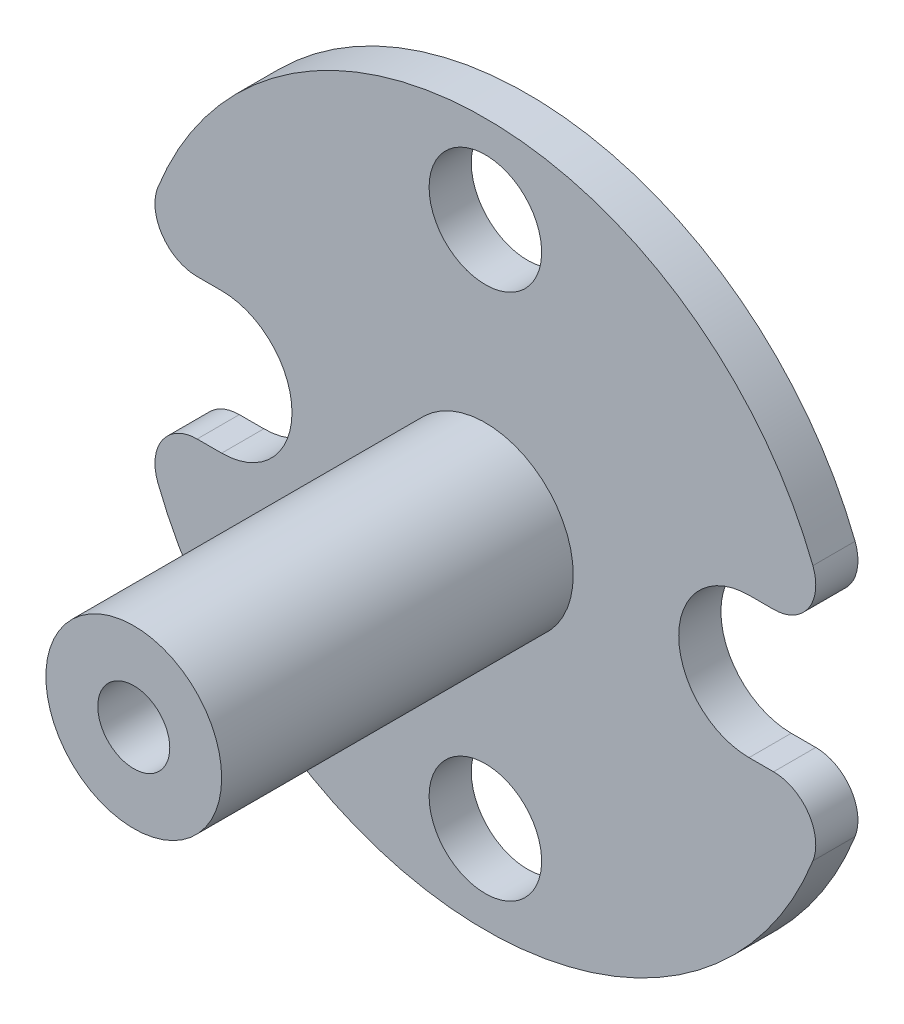
ISO-10303-21;
HEADER;
FILE_DESCRIPTION(('STEP AP214'),'2;1');
FILE_NAME('part.step','',(''),(''),'','','');
FILE_SCHEMA(('AUTOMOTIVE_DESIGN { 1 0 10303 214 1 1 1 1 }'));
ENDSEC;
DATA;
#1=APPLICATION_CONTEXT('core data for automotive mechanical design processes');
#2=APPLICATION_PROTOCOL_DEFINITION('international standard','automotive_design',2000,#1);
#3=PRODUCT_CONTEXT('',#1,'mechanical');
#4=PRODUCT('Part','Part','',(#3));
#5=PRODUCT_RELATED_PRODUCT_CATEGORY('part','',(#4));
#6=PRODUCT_DEFINITION_FORMATION('','',#4);
#7=PRODUCT_DEFINITION_CONTEXT('part definition',#1,'design');
#8=PRODUCT_DEFINITION('design','',#6,#7);
#9=PRODUCT_DEFINITION_SHAPE('','',#8);
#10=(LENGTH_UNIT() NAMED_UNIT(*) SI_UNIT(.MILLI.,.METRE.));
#11=(NAMED_UNIT(*) PLANE_ANGLE_UNIT() SI_UNIT($,.RADIAN.));
#12=(NAMED_UNIT(*) SI_UNIT($,.STERADIAN.) SOLID_ANGLE_UNIT());
#13=UNCERTAINTY_MEASURE_WITH_UNIT(LENGTH_MEASURE(1.E-05),#10,'distance_accuracy_value','');
#14=(GEOMETRIC_REPRESENTATION_CONTEXT(3) GLOBAL_UNCERTAINTY_ASSIGNED_CONTEXT((#13)) GLOBAL_UNIT_ASSIGNED_CONTEXT((#10,
#11,#12)) REPRESENTATION_CONTEXT('',''));
#15=CARTESIAN_POINT('',(0.,0.,0.));
#16=DIRECTION('',(0.,0.,1.));
#17=DIRECTION('',(1.,0.,0.));
#18=AXIS2_PLACEMENT_3D('',#15,#16,#17);
#19=CARTESIAN_POINT('',(-19.05,0.,3.048));
#20=DIRECTION('',(0.,0.,1.));
#21=DIRECTION('',(1.,0.,0.));
#22=AXIS2_PLACEMENT_3D('',#19,#20,#21);
#23=PLANE('',#22);
#24=CARTESIAN_POINT('',(0.,0.,3.048));
#25=DIRECTION('',(0.,0.,1.));
#26=DIRECTION('',(1.,0.,0.));
#27=AXIS2_PLACEMENT_3D('',#24,#25,#26);
#28=CIRCLE('',#27,6.35);
#29=CARTESIAN_POINT('',(6.35,0.,3.048));
#30=VERTEX_POINT('',#29);
#31=EDGE_CURVE('E147',#30,#30,#28,.T.);
#32=ORIENTED_EDGE('',*,*,#31,.F.);
#33=EDGE_LOOP('',(#32));
#34=FACE_BOUND('',#33,.T.);
#35=CARTESIAN_POINT('',(0.,19.05,3.048));
#36=DIRECTION('',(0.,0.,1.));
#37=DIRECTION('',(1.,0.,0.));
#38=AXIS2_PLACEMENT_3D('',#35,#36,#37);
#39=CIRCLE('',#38,4.065);
#40=CARTESIAN_POINT('',(-4.065,19.05,3.048));
#41=VERTEX_POINT('',#40);
#42=EDGE_CURVE('E168',#41,#41,#39,.T.);
#43=ORIENTED_EDGE('',*,*,#42,.F.);
#44=EDGE_LOOP('',(#43));
#45=FACE_BOUND('',#44,.T.);
#46=CARTESIAN_POINT('',(0.,0.,3.048));
#47=DIRECTION('',(0.,0.,1.));
#48=DIRECTION('',(1.,0.,0.));
#49=AXIS2_PLACEMENT_3D('',#46,#47,#48);
#50=CIRCLE('',#49,25.4);
#51=CARTESIAN_POINT('',(-23.6611408595794,-9.23636363636363,3.048));
#52=VERTEX_POINT('',#51);
#53=CARTESIAN_POINT('',(23.6611408595794,-9.23636363636363,3.048));
#54=VERTEX_POINT('',#53);
#55=EDGE_CURVE('E177',#52,#54,#50,.T.);
#56=ORIENTED_EDGE('',*,*,#55,.T.);
#57=CARTESIAN_POINT('',(20.8218039564299,-8.128,3.048));
#58=DIRECTION('',(0.,0.,1.));
#59=DIRECTION('',(1.,0.,0.));
#60=AXIS2_PLACEMENT_3D('',#57,#58,#59);
#61=CIRCLE('',#60,3.048);
#62=CARTESIAN_POINT('',(20.8218039564299,-5.08,3.048));
#63=VERTEX_POINT('',#62);
#64=EDGE_CURVE('E242',#54,#63,#61,.T.);
#65=ORIENTED_EDGE('',*,*,#64,.T.);
#66=DIRECTION('',(-1.,0.,0.));
#67=VECTOR('',#66,1.);
#68=CARTESIAN_POINT('',(19.05,-5.08,3.048));
#69=LINE('',#68,#67);
#70=CARTESIAN_POINT('',(19.05,-5.08,3.048));
#71=VERTEX_POINT('',#70);
#72=EDGE_CURVE('E185',#63,#71,#69,.T.);
#73=ORIENTED_EDGE('',*,*,#72,.T.);
#74=CARTESIAN_POINT('',(19.05,0.,3.048));
#75=DIRECTION('',(0.,0.,-1.));
#76=DIRECTION('',(-1.,0.,0.));
#77=AXIS2_PLACEMENT_3D('',#74,#75,#76);
#78=CIRCLE('',#77,5.08);
#79=CARTESIAN_POINT('',(19.05,5.08,3.048));
#80=VERTEX_POINT('',#79);
#81=EDGE_CURVE('E183',#71,#80,#78,.T.);
#82=ORIENTED_EDGE('',*,*,#81,.T.);
#83=DIRECTION('',(1.,0.,0.));
#84=VECTOR('',#83,1.);
#85=CARTESIAN_POINT('',(19.05,5.08,3.048));
#86=LINE('',#85,#84);
#87=CARTESIAN_POINT('',(20.8218039564299,5.08,3.048));
#88=VERTEX_POINT('',#87);
#89=EDGE_CURVE('E187',#80,#88,#86,.T.);
#90=ORIENTED_EDGE('',*,*,#89,.T.);
#91=CARTESIAN_POINT('',(20.8218039564299,8.128,3.048));
#92=DIRECTION('',(0.,0.,1.));
#93=DIRECTION('',(1.,0.,0.));
#94=AXIS2_PLACEMENT_3D('',#91,#92,#93);
#95=CIRCLE('',#94,3.048);
#96=CARTESIAN_POINT('',(23.6611408595794,9.23636363636363,3.048));
#97=VERTEX_POINT('',#96);
#98=EDGE_CURVE('E245',#88,#97,#95,.T.);
#99=ORIENTED_EDGE('',*,*,#98,.T.);
#100=CARTESIAN_POINT('',(0.,0.,3.048));
#101=DIRECTION('',(0.,0.,1.));
#102=DIRECTION('',(1.,0.,0.));
#103=AXIS2_PLACEMENT_3D('',#100,#101,#102);
#104=CIRCLE('',#103,25.4);
#105=CARTESIAN_POINT('',(-23.6611408595794,9.23636363636363,3.048));
#106=VERTEX_POINT('',#105);
#107=EDGE_CURVE('E186',#97,#106,#104,.T.);
#108=ORIENTED_EDGE('',*,*,#107,.T.);
#109=CARTESIAN_POINT('',(-20.8218039564299,8.128,3.048));
#110=DIRECTION('',(0.,0.,1.));
#111=DIRECTION('',(1.,0.,0.));
#112=AXIS2_PLACEMENT_3D('',#109,#110,#111);
#113=CIRCLE('',#112,3.048);
#114=CARTESIAN_POINT('',(-20.8218039564299,5.08,3.048));
#115=VERTEX_POINT('',#114);
#116=EDGE_CURVE('E58',#106,#115,#113,.T.);
#117=ORIENTED_EDGE('',*,*,#116,.T.);
#118=DIRECTION('',(1.,0.,0.));
#119=VECTOR('',#118,1.);
#120=CARTESIAN_POINT('',(-19.05,5.08,3.048));
#121=LINE('',#120,#119);
#122=CARTESIAN_POINT('',(-19.05,5.08,3.048));
#123=VERTEX_POINT('',#122);
#124=EDGE_CURVE('E192',#115,#123,#121,.T.);
#125=ORIENTED_EDGE('',*,*,#124,.T.);
#126=CARTESIAN_POINT('',(-19.05,0.,3.048));
#127=DIRECTION('',(0.,0.,-1.));
#128=DIRECTION('',(1.,0.,0.));
#129=AXIS2_PLACEMENT_3D('',#126,#127,#128);
#130=CIRCLE('',#129,5.08);
#131=CARTESIAN_POINT('',(-19.05,-5.08,3.048));
#132=VERTEX_POINT('',#131);
#133=EDGE_CURVE('E175',#123,#132,#130,.T.);
#134=ORIENTED_EDGE('',*,*,#133,.T.);
#135=DIRECTION('',(-1.,0.,0.));
#136=VECTOR('',#135,1.);
#137=CARTESIAN_POINT('',(-19.05,-5.08,3.048));
#138=LINE('',#137,#136);
#139=CARTESIAN_POINT('',(-20.8218039564299,-5.08,3.048));
#140=VERTEX_POINT('',#139);
#141=EDGE_CURVE('E174',#132,#140,#138,.T.);
#142=ORIENTED_EDGE('',*,*,#141,.T.);
#143=CARTESIAN_POINT('',(-20.8218039564299,-8.128,3.048));
#144=DIRECTION('',(0.,0.,1.));
#145=DIRECTION('',(1.,0.,0.));
#146=AXIS2_PLACEMENT_3D('',#143,#144,#145);
#147=CIRCLE('',#146,3.048);
#148=EDGE_CURVE('E237',#140,#52,#147,.T.);
#149=ORIENTED_EDGE('',*,*,#148,.T.);
#150=EDGE_LOOP('',(#56,#65,#73,#82,#90,#99,#108,#117,#125,#134,#142,#149));
#151=FACE_BOUND('',#150,.T.);
#152=CARTESIAN_POINT('',(0.,-19.05,3.048));
#153=DIRECTION('',(0.,0.,1.));
#154=DIRECTION('',(1.,0.,0.));
#155=AXIS2_PLACEMENT_3D('',#152,#153,#154);
#156=CIRCLE('',#155,4.065);
#157=CARTESIAN_POINT('',(-4.065,-19.05,3.048));
#158=VERTEX_POINT('',#157);
#159=EDGE_CURVE('E160',#158,#158,#156,.T.);
#160=ORIENTED_EDGE('',*,*,#159,.F.);
#161=EDGE_LOOP('',(#160));
#162=FACE_BOUND('',#161,.T.);
#163=ADVANCED_FACE('F44',(#34,#45,#151,#162),#23,.T.);
#164=CARTESIAN_POINT('',(-19.05,0.,0.));
#165=DIRECTION('',(0.,0.,1.));
#166=DIRECTION('',(1.,0.,0.));
#167=AXIS2_PLACEMENT_3D('',#164,#165,#166);
#168=PLANE('',#167);
#169=DIRECTION('',(-1.,0.,0.));
#170=VECTOR('',#169,1.);
#171=CARTESIAN_POINT('',(19.05,-5.08,0.));
#172=LINE('',#171,#170);
#173=CARTESIAN_POINT('',(20.8218039564299,-5.08,0.));
#174=VERTEX_POINT('',#173);
#175=CARTESIAN_POINT('',(19.05,-5.08,0.));
#176=VERTEX_POINT('',#175);
#177=EDGE_CURVE('E202',#174,#176,#172,.T.);
#178=ORIENTED_EDGE('',*,*,#177,.F.);
#179=CARTESIAN_POINT('',(20.8218039564299,-8.128,0.));
#180=DIRECTION('',(0.,0.,1.));
#181=DIRECTION('',(1.,0.,0.));
#182=AXIS2_PLACEMENT_3D('',#179,#180,#181);
#183=CIRCLE('',#182,3.048);
#184=CARTESIAN_POINT('',(23.6611408595794,-9.23636363636363,0.));
#185=VERTEX_POINT('',#184);
#186=EDGE_CURVE('E235',#174,#185,#183,.F.);
#187=ORIENTED_EDGE('',*,*,#186,.T.);
#188=CARTESIAN_POINT('',(0.,0.,0.));
#189=DIRECTION('',(0.,0.,1.));
#190=DIRECTION('',(1.,0.,0.));
#191=AXIS2_PLACEMENT_3D('',#188,#189,#190);
#192=CIRCLE('',#191,25.4);
#193=CARTESIAN_POINT('',(-23.6611408595794,-9.23636363636363,0.));
#194=VERTEX_POINT('',#193);
#195=EDGE_CURVE('E198',#194,#185,#192,.T.);
#196=ORIENTED_EDGE('',*,*,#195,.F.);
#197=CARTESIAN_POINT('',(-20.8218039564299,-8.128,0.));
#198=DIRECTION('',(0.,0.,1.));
#199=DIRECTION('',(1.,0.,0.));
#200=AXIS2_PLACEMENT_3D('',#197,#198,#199);
#201=CIRCLE('',#200,3.048);
#202=CARTESIAN_POINT('',(-20.8218039564299,-5.08,0.));
#203=VERTEX_POINT('',#202);
#204=EDGE_CURVE('E228',#194,#203,#201,.F.);
#205=ORIENTED_EDGE('',*,*,#204,.T.);
#206=DIRECTION('',(-1.,0.,0.));
#207=VECTOR('',#206,1.);
#208=CARTESIAN_POINT('',(-19.05,-5.08,0.));
#209=LINE('',#208,#207);
#210=CARTESIAN_POINT('',(-19.05,-5.08,0.));
#211=VERTEX_POINT('',#210);
#212=EDGE_CURVE('E196',#211,#203,#209,.T.);
#213=ORIENTED_EDGE('',*,*,#212,.F.);
#214=CARTESIAN_POINT('',(-19.05,0.,0.));
#215=DIRECTION('',(0.,0.,-1.));
#216=DIRECTION('',(1.,0.,0.));
#217=AXIS2_PLACEMENT_3D('',#214,#215,#216);
#218=CIRCLE('',#217,5.08);
#219=CARTESIAN_POINT('',(-19.05,5.08,0.));
#220=VERTEX_POINT('',#219);
#221=EDGE_CURVE('E169',#220,#211,#218,.T.);
#222=ORIENTED_EDGE('',*,*,#221,.F.);
#223=DIRECTION('',(1.,0.,0.));
#224=VECTOR('',#223,1.);
#225=CARTESIAN_POINT('',(-19.05,5.08,0.));
#226=LINE('',#225,#224);
#227=CARTESIAN_POINT('',(-20.8218039564299,5.08,0.));
#228=VERTEX_POINT('',#227);
#229=EDGE_CURVE('E176',#228,#220,#226,.T.);
#230=ORIENTED_EDGE('',*,*,#229,.F.);
#231=CARTESIAN_POINT('',(-20.8218039564299,8.128,0.));
#232=DIRECTION('',(0.,0.,1.));
#233=DIRECTION('',(1.,0.,0.));
#234=AXIS2_PLACEMENT_3D('',#231,#232,#233);
#235=CIRCLE('',#234,3.048);
#236=CARTESIAN_POINT('',(-23.6611408595794,9.23636363636363,0.));
#237=VERTEX_POINT('',#236);
#238=EDGE_CURVE('E226',#228,#237,#235,.F.);
#239=ORIENTED_EDGE('',*,*,#238,.T.);
#240=CARTESIAN_POINT('',(0.,0.,0.));
#241=DIRECTION('',(0.,0.,1.));
#242=DIRECTION('',(1.,0.,0.));
#243=AXIS2_PLACEMENT_3D('',#240,#241,#242);
#244=CIRCLE('',#243,25.4);
#245=CARTESIAN_POINT('',(23.6611408595794,9.23636363636363,0.));
#246=VERTEX_POINT('',#245);
#247=EDGE_CURVE('E209',#246,#237,#244,.T.);
#248=ORIENTED_EDGE('',*,*,#247,.F.);
#249=CARTESIAN_POINT('',(20.8218039564299,8.128,0.));
#250=DIRECTION('',(0.,0.,1.));
#251=DIRECTION('',(1.,0.,0.));
#252=AXIS2_PLACEMENT_3D('',#249,#250,#251);
#253=CIRCLE('',#252,3.048);
#254=CARTESIAN_POINT('',(20.8218039564299,5.08,0.));
#255=VERTEX_POINT('',#254);
#256=EDGE_CURVE('E229',#246,#255,#253,.F.);
#257=ORIENTED_EDGE('',*,*,#256,.T.);
#258=DIRECTION('',(1.,0.,0.));
#259=VECTOR('',#258,1.);
#260=CARTESIAN_POINT('',(19.05,5.08,0.));
#261=LINE('',#260,#259);
#262=CARTESIAN_POINT('',(19.05,5.08,0.));
#263=VERTEX_POINT('',#262);
#264=EDGE_CURVE('E207',#263,#255,#261,.T.);
#265=ORIENTED_EDGE('',*,*,#264,.F.);
#266=CARTESIAN_POINT('',(19.05,0.,0.));
#267=DIRECTION('',(0.,0.,-1.));
#268=DIRECTION('',(-1.,0.,0.));
#269=AXIS2_PLACEMENT_3D('',#266,#267,#268);
#270=CIRCLE('',#269,5.08);
#271=EDGE_CURVE('E203',#176,#263,#270,.T.);
#272=ORIENTED_EDGE('',*,*,#271,.F.);
#273=EDGE_LOOP('',(#178,#187,#196,#205,#213,#222,#230,#239,#248,#257,#265,#272));
#274=FACE_BOUND('',#273,.T.);
#275=CARTESIAN_POINT('',(0.,19.05,0.));
#276=DIRECTION('',(0.,0.,1.));
#277=DIRECTION('',(1.,0.,0.));
#278=AXIS2_PLACEMENT_3D('',#275,#276,#277);
#279=CIRCLE('',#278,4.065);
#280=CARTESIAN_POINT('',(-4.065,19.05,0.));
#281=VERTEX_POINT('',#280);
#282=EDGE_CURVE('E161',#281,#281,#279,.T.);
#283=ORIENTED_EDGE('',*,*,#282,.T.);
#284=EDGE_LOOP('',(#283));
#285=FACE_BOUND('',#284,.T.);
#286=CARTESIAN_POINT('',(0.,-19.05,0.));
#287=DIRECTION('',(0.,0.,1.));
#288=DIRECTION('',(1.,0.,0.));
#289=AXIS2_PLACEMENT_3D('',#286,#287,#288);
#290=CIRCLE('',#289,4.065);
#291=CARTESIAN_POINT('',(-4.065,-19.05,0.));
#292=VERTEX_POINT('',#291);
#293=EDGE_CURVE('E159',#292,#292,#290,.T.);
#294=ORIENTED_EDGE('',*,*,#293,.T.);
#295=EDGE_LOOP('',(#294));
#296=FACE_BOUND('',#295,.T.);
#297=ADVANCED_FACE('F261',(#274,#285,#296),#168,.F.);
#298=CARTESIAN_POINT('',(-19.05,0.,3.048));
#299=DIRECTION('',(0.,0.,-1.));
#300=DIRECTION('',(-1.,0.,0.));
#301=AXIS2_PLACEMENT_3D('',#298,#299,#300);
#302=CYLINDRICAL_SURFACE('',#301,5.08);
#303=ORIENTED_EDGE('',*,*,#221,.T.);
#304=DIRECTION('',(0.,0.,-1.));
#305=VECTOR('',#304,1.);
#306=CARTESIAN_POINT('',(-19.05,-5.08,3.048));
#307=LINE('',#306,#305);
#308=EDGE_CURVE('E220',#132,#211,#307,.T.);
#309=ORIENTED_EDGE('',*,*,#308,.F.);
#310=ORIENTED_EDGE('',*,*,#133,.F.);
#311=DIRECTION('',(0.,0.,-1.));
#312=VECTOR('',#311,1.);
#313=CARTESIAN_POINT('',(-19.05,5.08,3.048));
#314=LINE('',#313,#312);
#315=EDGE_CURVE('E194',#123,#220,#314,.T.);
#316=ORIENTED_EDGE('',*,*,#315,.T.);
#317=EDGE_LOOP('',(#303,#309,#310,#316));
#318=FACE_BOUND('',#317,.T.);
#319=ADVANCED_FACE('F266',(#318),#302,.F.);
#320=CARTESIAN_POINT('',(-19.05,-5.08,3.048));
#321=DIRECTION('',(0.,-1.,0.));
#322=DIRECTION('',(0.,0.,-1.));
#323=AXIS2_PLACEMENT_3D('',#320,#321,#322);
#324=PLANE('',#323);
#325=ORIENTED_EDGE('',*,*,#212,.T.);
#326=DIRECTION('',(0.,0.,-1.));
#327=VECTOR('',#326,1.);
#328=CARTESIAN_POINT('',(-20.8218039564299,-5.08,3.048));
#329=LINE('',#328,#327);
#330=EDGE_CURVE('E11',#203,#140,#329,.F.);
#331=ORIENTED_EDGE('',*,*,#330,.T.);
#332=ORIENTED_EDGE('',*,*,#141,.F.);
#333=ORIENTED_EDGE('',*,*,#308,.T.);
#334=EDGE_LOOP('',(#325,#331,#332,#333));
#335=FACE_BOUND('',#334,.T.);
#336=ADVANCED_FACE('F337',(#335),#324,.F.);
#337=CARTESIAN_POINT('',(0.,0.,3.048));
#338=DIRECTION('',(0.,0.,-1.));
#339=DIRECTION('',(-1.,0.,0.));
#340=AXIS2_PLACEMENT_3D('',#337,#338,#339);
#341=CYLINDRICAL_SURFACE('',#340,25.4);
#342=ORIENTED_EDGE('',*,*,#195,.T.);
#343=DIRECTION('',(0.,0.,-1.));
#344=VECTOR('',#343,1.);
#345=CARTESIAN_POINT('',(23.6611408595794,-9.23636363636363,3.048));
#346=LINE('',#345,#344);
#347=EDGE_CURVE('E240',#185,#54,#346,.F.);
#348=ORIENTED_EDGE('',*,*,#347,.T.);
#349=ORIENTED_EDGE('',*,*,#55,.F.);
#350=DIRECTION('',(0.,0.,-1.));
#351=VECTOR('',#350,1.);
#352=CARTESIAN_POINT('',(-23.6611408595794,-9.23636363636363,3.048));
#353=LINE('',#352,#351);
#354=EDGE_CURVE('E234',#52,#194,#353,.T.);
#355=ORIENTED_EDGE('',*,*,#354,.T.);
#356=EDGE_LOOP('',(#342,#348,#349,#355));
#357=FACE_BOUND('',#356,.T.);
#358=ADVANCED_FACE('F280',(#357),#341,.T.);
#359=CARTESIAN_POINT('',(19.05,-5.08,3.048));
#360=DIRECTION('',(0.,-1.,0.));
#361=DIRECTION('',(0.,0.,-1.));
#362=AXIS2_PLACEMENT_3D('',#359,#360,#361);
#363=PLANE('',#362);
#364=ORIENTED_EDGE('',*,*,#72,.F.);
#365=DIRECTION('',(0.,0.,-1.));
#366=VECTOR('',#365,1.);
#367=CARTESIAN_POINT('',(20.8218039564299,-5.08,3.048));
#368=LINE('',#367,#366);
#369=EDGE_CURVE('E224',#63,#174,#368,.T.);
#370=ORIENTED_EDGE('',*,*,#369,.T.);
#371=ORIENTED_EDGE('',*,*,#177,.T.);
#372=DIRECTION('',(0.,0.,-1.));
#373=VECTOR('',#372,1.);
#374=CARTESIAN_POINT('',(19.05,-5.08,3.048));
#375=LINE('',#374,#373);
#376=EDGE_CURVE('E217',#71,#176,#375,.T.);
#377=ORIENTED_EDGE('',*,*,#376,.F.);
#378=EDGE_LOOP('',(#364,#370,#371,#377));
#379=FACE_BOUND('',#378,.T.);
#380=ADVANCED_FACE('F286',(#379),#363,.F.);
#381=CARTESIAN_POINT('',(19.05,0.,3.048));
#382=DIRECTION('',(0.,0.,-1.));
#383=DIRECTION('',(-1.,0.,0.));
#384=AXIS2_PLACEMENT_3D('',#381,#382,#383);
#385=CYLINDRICAL_SURFACE('',#384,5.08);
#386=ORIENTED_EDGE('',*,*,#271,.T.);
#387=DIRECTION('',(0.,0.,-1.));
#388=VECTOR('',#387,1.);
#389=CARTESIAN_POINT('',(19.05,5.08,3.048));
#390=LINE('',#389,#388);
#391=EDGE_CURVE('E211',#80,#263,#390,.T.);
#392=ORIENTED_EDGE('',*,*,#391,.F.);
#393=ORIENTED_EDGE('',*,*,#81,.F.);
#394=ORIENTED_EDGE('',*,*,#376,.T.);
#395=EDGE_LOOP('',(#386,#392,#393,#394));
#396=FACE_BOUND('',#395,.T.);
#397=ADVANCED_FACE('F291',(#396),#385,.F.);
#398=CARTESIAN_POINT('',(19.05,5.08,3.048));
#399=DIRECTION('',(0.,1.,0.));
#400=DIRECTION('',(0.,0.,1.));
#401=AXIS2_PLACEMENT_3D('',#398,#399,#400);
#402=PLANE('',#401);
#403=ORIENTED_EDGE('',*,*,#264,.T.);
#404=DIRECTION('',(0.,0.,-1.));
#405=VECTOR('',#404,1.);
#406=CARTESIAN_POINT('',(20.8218039564299,5.08,3.048));
#407=LINE('',#406,#405);
#408=EDGE_CURVE('E249',#255,#88,#407,.F.);
#409=ORIENTED_EDGE('',*,*,#408,.T.);
#410=ORIENTED_EDGE('',*,*,#89,.F.);
#411=ORIENTED_EDGE('',*,*,#391,.T.);
#412=EDGE_LOOP('',(#403,#409,#410,#411));
#413=FACE_BOUND('',#412,.T.);
#414=ADVANCED_FACE('F298',(#413),#402,.F.);
#415=CARTESIAN_POINT('',(0.,0.,3.048));
#416=DIRECTION('',(0.,0.,-1.));
#417=DIRECTION('',(-1.,0.,0.));
#418=AXIS2_PLACEMENT_3D('',#415,#416,#417);
#419=CYLINDRICAL_SURFACE('',#418,25.4);
#420=ORIENTED_EDGE('',*,*,#107,.F.);
#421=DIRECTION('',(0.,0.,-1.));
#422=VECTOR('',#421,1.);
#423=CARTESIAN_POINT('',(23.6611408595794,9.23636363636363,3.048));
#424=LINE('',#423,#422);
#425=EDGE_CURVE('E250',#97,#246,#424,.T.);
#426=ORIENTED_EDGE('',*,*,#425,.T.);
#427=ORIENTED_EDGE('',*,*,#247,.T.);
#428=DIRECTION('',(0.,0.,-1.));
#429=VECTOR('',#428,1.);
#430=CARTESIAN_POINT('',(-23.6611408595794,9.23636363636363,3.048));
#431=LINE('',#430,#429);
#432=EDGE_CURVE('E69',#237,#106,#431,.F.);
#433=ORIENTED_EDGE('',*,*,#432,.T.);
#434=EDGE_LOOP('',(#420,#426,#427,#433));
#435=FACE_BOUND('',#434,.T.);
#436=ADVANCED_FACE('F301',(#435),#419,.T.);
#437=CARTESIAN_POINT('',(-19.05,5.08,3.048));
#438=DIRECTION('',(0.,1.,0.));
#439=DIRECTION('',(0.,0.,1.));
#440=AXIS2_PLACEMENT_3D('',#437,#438,#439);
#441=PLANE('',#440);
#442=ORIENTED_EDGE('',*,*,#124,.F.);
#443=DIRECTION('',(0.,0.,-1.));
#444=VECTOR('',#443,1.);
#445=CARTESIAN_POINT('',(-20.8218039564299,5.08,3.048));
#446=LINE('',#445,#444);
#447=EDGE_CURVE('E52',#115,#228,#446,.T.);
#448=ORIENTED_EDGE('',*,*,#447,.T.);
#449=ORIENTED_EDGE('',*,*,#229,.T.);
#450=ORIENTED_EDGE('',*,*,#315,.F.);
#451=EDGE_LOOP('',(#442,#448,#449,#450));
#452=FACE_BOUND('',#451,.T.);
#453=ADVANCED_FACE('F253',(#452),#441,.F.);
#454=CARTESIAN_POINT('',(0.,19.05,3.048));
#455=DIRECTION('',(0.,0.,-1.));
#456=DIRECTION('',(-1.,0.,0.));
#457=AXIS2_PLACEMENT_3D('',#454,#455,#456);
#458=CYLINDRICAL_SURFACE('',#457,4.065);
#459=CARTESIAN_POINT('',(-4.065,19.05,3.048));
#460=CARTESIAN_POINT('',(-4.065,19.05,3.01625));
#461=CARTESIAN_POINT('',(-4.065,19.05,2.9845));
#462=CARTESIAN_POINT('',(-4.065,19.05,2.921));
#463=CARTESIAN_POINT('',(-4.065,19.05,2.88925));
#464=CARTESIAN_POINT('',(-4.065,19.05,2.82575));
#465=CARTESIAN_POINT('',(-4.065,19.05,2.794));
#466=CARTESIAN_POINT('',(-4.065,19.05,2.7305));
#467=CARTESIAN_POINT('',(-4.065,19.05,2.69875));
#468=CARTESIAN_POINT('',(-4.065,19.05,2.63525));
#469=CARTESIAN_POINT('',(-4.065,19.05,2.6035));
#470=CARTESIAN_POINT('',(-4.065,19.05,2.54));
#471=CARTESIAN_POINT('',(-4.065,19.05,2.50825));
#472=CARTESIAN_POINT('',(-4.065,19.05,2.44475));
#473=CARTESIAN_POINT('',(-4.065,19.05,2.413));
#474=CARTESIAN_POINT('',(-4.065,19.05,2.3495));
#475=CARTESIAN_POINT('',(-4.065,19.05,2.31775));
#476=CARTESIAN_POINT('',(-4.065,19.05,2.25425));
#477=CARTESIAN_POINT('',(-4.065,19.05,2.2225));
#478=CARTESIAN_POINT('',(-4.065,19.05,2.159));
#479=CARTESIAN_POINT('',(-4.065,19.05,2.12725));
#480=CARTESIAN_POINT('',(-4.065,19.05,2.06375));
#481=CARTESIAN_POINT('',(-4.065,19.05,2.032));
#482=CARTESIAN_POINT('',(-4.065,19.05,1.9685));
#483=CARTESIAN_POINT('',(-4.065,19.05,1.93675));
#484=CARTESIAN_POINT('',(-4.065,19.05,1.87325));
#485=CARTESIAN_POINT('',(-4.065,19.05,1.8415));
#486=CARTESIAN_POINT('',(-4.065,19.05,1.778));
#487=CARTESIAN_POINT('',(-4.065,19.05,1.74625));
#488=CARTESIAN_POINT('',(-4.065,19.05,1.68275));
#489=CARTESIAN_POINT('',(-4.065,19.05,1.651));
#490=CARTESIAN_POINT('',(-4.065,19.05,1.5875));
#491=CARTESIAN_POINT('',(-4.065,19.05,1.55575));
#492=CARTESIAN_POINT('',(-4.065,19.05,1.49225));
#493=CARTESIAN_POINT('',(-4.065,19.05,1.4605));
#494=CARTESIAN_POINT('',(-4.065,19.05,1.397));
#495=CARTESIAN_POINT('',(-4.065,19.05,1.36525));
#496=CARTESIAN_POINT('',(-4.065,19.05,1.30175));
#497=CARTESIAN_POINT('',(-4.065,19.05,1.27));
#498=CARTESIAN_POINT('',(-4.065,19.05,1.2065));
#499=CARTESIAN_POINT('',(-4.065,19.05,1.17475));
#500=CARTESIAN_POINT('',(-4.065,19.05,1.11125));
#501=CARTESIAN_POINT('',(-4.065,19.05,1.0795));
#502=CARTESIAN_POINT('',(-4.065,19.05,1.016));
#503=CARTESIAN_POINT('',(-4.065,19.05,0.98425));
#504=CARTESIAN_POINT('',(-4.065,19.05,0.92075));
#505=CARTESIAN_POINT('',(-4.065,19.05,0.889));
#506=CARTESIAN_POINT('',(-4.065,19.05,0.8255));
#507=CARTESIAN_POINT('',(-4.065,19.05,0.79375));
#508=CARTESIAN_POINT('',(-4.065,19.05,0.73025));
#509=CARTESIAN_POINT('',(-4.065,19.05,0.6985));
#510=CARTESIAN_POINT('',(-4.065,19.05,0.635));
#511=CARTESIAN_POINT('',(-4.065,19.05,0.60325));
#512=CARTESIAN_POINT('',(-4.065,19.05,0.53975));
#513=CARTESIAN_POINT('',(-4.065,19.05,0.508));
#514=CARTESIAN_POINT('',(-4.065,19.05,0.4445));
#515=CARTESIAN_POINT('',(-4.065,19.05,0.41275));
#516=CARTESIAN_POINT('',(-4.065,19.05,0.34925));
#517=CARTESIAN_POINT('',(-4.065,19.05,0.3175));
#518=CARTESIAN_POINT('',(-4.065,19.05,0.254));
#519=CARTESIAN_POINT('',(-4.065,19.05,0.22225));
#520=CARTESIAN_POINT('',(-4.065,19.05,0.15875));
#521=CARTESIAN_POINT('',(-4.065,19.05,0.127));
#522=CARTESIAN_POINT('',(-4.065,19.05,0.0634999999999999));
#523=CARTESIAN_POINT('',(-4.065,19.05,0.03175));
#524=CARTESIAN_POINT('',(-4.065,19.05,0.));
#525=B_SPLINE_CURVE_WITH_KNOTS('',3,(#459,#460,#461,#462,#463,#464,#465,#466,#467,#468,#469,
#470,#471,#472,#473,#474,#475,#476,#477,#478,#479,#480,#481,#482,#483,#484,#485,#486,#487,#488,
#489,#490,#491,#492,#493,#494,#495,#496,#497,#498,#499,#500,#501,#502,#503,#504,#505,#506,#507,
#508,#509,#510,#511,#512,#513,#514,#515,#516,#517,#518,#519,#520,#521,#522,#523,#524),
.UNSPECIFIED.,.F.,.F.,(4,2,2,2,2,2,2,2,2,2,2,2,2,2,2,2,2,2,2,2,2,2,2,2,2,2,2,2,2,2,2,2,4),(0.,
0.0952500000000003,0.1905,0.28575,0.381,0.47625,0.5715,0.66675,0.762,0.85725,0.9525,1.04775,
1.143,1.23825,1.3335,1.42875,1.524,1.61925,1.7145,1.80975,1.905,2.00025,2.0955,2.19075,2.286,
2.38125,2.4765,2.57175,2.667,2.76225,2.8575,2.95275,3.048),.UNSPECIFIED.);
#526=EDGE_CURVE('BSEAM322',#41,#281,#525,.T.);
#527=ORIENTED_EDGE('',*,*,#42,.T.);
#528=ORIENTED_EDGE('',*,*,#282,.F.);
#529=ORIENTED_EDGE('',*,*,#526,.T.);
#530=ORIENTED_EDGE('',*,*,#526,.F.);
#531=EDGE_LOOP('',(#527,#529,#528,#530));
#532=FACE_BOUND('',#531,.T.);
#533=ADVANCED_FACE('F322',(#532),#458,.F.);
#534=CARTESIAN_POINT('',(0.,-19.05,3.048));
#535=DIRECTION('',(0.,0.,-1.));
#536=DIRECTION('',(-1.,0.,0.));
#537=AXIS2_PLACEMENT_3D('',#534,#535,#536);
#538=CYLINDRICAL_SURFACE('',#537,4.065);
#539=CARTESIAN_POINT('',(-4.065,-19.05,3.048));
#540=CARTESIAN_POINT('',(-4.065,-19.05,3.01625));
#541=CARTESIAN_POINT('',(-4.065,-19.05,2.9845));
#542=CARTESIAN_POINT('',(-4.065,-19.05,2.921));
#543=CARTESIAN_POINT('',(-4.065,-19.05,2.88925));
#544=CARTESIAN_POINT('',(-4.065,-19.05,2.82575));
#545=CARTESIAN_POINT('',(-4.065,-19.05,2.794));
#546=CARTESIAN_POINT('',(-4.065,-19.05,2.7305));
#547=CARTESIAN_POINT('',(-4.065,-19.05,2.69875));
#548=CARTESIAN_POINT('',(-4.065,-19.05,2.63525));
#549=CARTESIAN_POINT('',(-4.065,-19.05,2.6035));
#550=CARTESIAN_POINT('',(-4.065,-19.05,2.54));
#551=CARTESIAN_POINT('',(-4.065,-19.05,2.50825));
#552=CARTESIAN_POINT('',(-4.065,-19.05,2.44475));
#553=CARTESIAN_POINT('',(-4.065,-19.05,2.413));
#554=CARTESIAN_POINT('',(-4.065,-19.05,2.3495));
#555=CARTESIAN_POINT('',(-4.065,-19.05,2.31775));
#556=CARTESIAN_POINT('',(-4.065,-19.05,2.25425));
#557=CARTESIAN_POINT('',(-4.065,-19.05,2.2225));
#558=CARTESIAN_POINT('',(-4.065,-19.05,2.159));
#559=CARTESIAN_POINT('',(-4.065,-19.05,2.12725));
#560=CARTESIAN_POINT('',(-4.065,-19.05,2.06375));
#561=CARTESIAN_POINT('',(-4.065,-19.05,2.032));
#562=CARTESIAN_POINT('',(-4.065,-19.05,1.9685));
#563=CARTESIAN_POINT('',(-4.065,-19.05,1.93675));
#564=CARTESIAN_POINT('',(-4.065,-19.05,1.87325));
#565=CARTESIAN_POINT('',(-4.065,-19.05,1.8415));
#566=CARTESIAN_POINT('',(-4.065,-19.05,1.778));
#567=CARTESIAN_POINT('',(-4.065,-19.05,1.74625));
#568=CARTESIAN_POINT('',(-4.065,-19.05,1.68275));
#569=CARTESIAN_POINT('',(-4.065,-19.05,1.651));
#570=CARTESIAN_POINT('',(-4.065,-19.05,1.5875));
#571=CARTESIAN_POINT('',(-4.065,-19.05,1.55575));
#572=CARTESIAN_POINT('',(-4.065,-19.05,1.49225));
#573=CARTESIAN_POINT('',(-4.065,-19.05,1.4605));
#574=CARTESIAN_POINT('',(-4.065,-19.05,1.397));
#575=CARTESIAN_POINT('',(-4.065,-19.05,1.36525));
#576=CARTESIAN_POINT('',(-4.065,-19.05,1.30175));
#577=CARTESIAN_POINT('',(-4.065,-19.05,1.27));
#578=CARTESIAN_POINT('',(-4.065,-19.05,1.2065));
#579=CARTESIAN_POINT('',(-4.065,-19.05,1.17475));
#580=CARTESIAN_POINT('',(-4.065,-19.05,1.11125));
#581=CARTESIAN_POINT('',(-4.065,-19.05,1.0795));
#582=CARTESIAN_POINT('',(-4.065,-19.05,1.016));
#583=CARTESIAN_POINT('',(-4.065,-19.05,0.98425));
#584=CARTESIAN_POINT('',(-4.065,-19.05,0.92075));
#585=CARTESIAN_POINT('',(-4.065,-19.05,0.889));
#586=CARTESIAN_POINT('',(-4.065,-19.05,0.8255));
#587=CARTESIAN_POINT('',(-4.065,-19.05,0.79375));
#588=CARTESIAN_POINT('',(-4.065,-19.05,0.73025));
#589=CARTESIAN_POINT('',(-4.065,-19.05,0.6985));
#590=CARTESIAN_POINT('',(-4.065,-19.05,0.635));
#591=CARTESIAN_POINT('',(-4.065,-19.05,0.60325));
#592=CARTESIAN_POINT('',(-4.065,-19.05,0.53975));
#593=CARTESIAN_POINT('',(-4.065,-19.05,0.508));
#594=CARTESIAN_POINT('',(-4.065,-19.05,0.4445));
#595=CARTESIAN_POINT('',(-4.065,-19.05,0.41275));
#596=CARTESIAN_POINT('',(-4.065,-19.05,0.34925));
#597=CARTESIAN_POINT('',(-4.065,-19.05,0.3175));
#598=CARTESIAN_POINT('',(-4.065,-19.05,0.254));
#599=CARTESIAN_POINT('',(-4.065,-19.05,0.22225));
#600=CARTESIAN_POINT('',(-4.065,-19.05,0.15875));
#601=CARTESIAN_POINT('',(-4.065,-19.05,0.127));
#602=CARTESIAN_POINT('',(-4.065,-19.05,0.0634999999999999));
#603=CARTESIAN_POINT('',(-4.065,-19.05,0.03175));
#604=CARTESIAN_POINT('',(-4.065,-19.05,0.));
#605=B_SPLINE_CURVE_WITH_KNOTS('',3,(#539,#540,#541,#542,#543,#544,#545,#546,#547,#548,#549,
#550,#551,#552,#553,#554,#555,#556,#557,#558,#559,#560,#561,#562,#563,#564,#565,#566,#567,#568,
#569,#570,#571,#572,#573,#574,#575,#576,#577,#578,#579,#580,#581,#582,#583,#584,#585,#586,#587,
#588,#589,#590,#591,#592,#593,#594,#595,#596,#597,#598,#599,#600,#601,#602,#603,#604),
.UNSPECIFIED.,.F.,.F.,(4,2,2,2,2,2,2,2,2,2,2,2,2,2,2,2,2,2,2,2,2,2,2,2,2,2,2,2,2,2,2,2,4),(0.,
0.0952500000000003,0.1905,0.28575,0.381,0.47625,0.5715,0.66675,0.762,0.85725,0.9525,1.04775,
1.143,1.23825,1.3335,1.42875,1.524,1.61925,1.7145,1.80975,1.905,2.00025,2.0955,2.19075,2.286,
2.38125,2.4765,2.57175,2.667,2.76225,2.8575,2.95275,3.048),.UNSPECIFIED.);
#606=EDGE_CURVE('BSEAM345',#158,#292,#605,.T.);
#607=ORIENTED_EDGE('',*,*,#159,.T.);
#608=ORIENTED_EDGE('',*,*,#293,.F.);
#609=ORIENTED_EDGE('',*,*,#606,.T.);
#610=ORIENTED_EDGE('',*,*,#606,.F.);
#611=EDGE_LOOP('',(#607,#609,#608,#610));
#612=FACE_BOUND('',#611,.T.);
#613=ADVANCED_FACE('F345',(#612),#538,.F.);
#614=CARTESIAN_POINT('',(20.8218039564299,-8.128,3.048));
#615=DIRECTION('',(0.,0.,-1.));
#616=DIRECTION('',(-1.,0.,0.));
#617=AXIS2_PLACEMENT_3D('',#614,#615,#616);
#618=CYLINDRICAL_SURFACE('',#617,3.048);
#619=ORIENTED_EDGE('',*,*,#64,.F.);
#620=ORIENTED_EDGE('',*,*,#347,.F.);
#621=ORIENTED_EDGE('',*,*,#186,.F.);
#622=ORIENTED_EDGE('',*,*,#369,.F.);
#623=EDGE_LOOP('',(#619,#620,#621,#622));
#624=FACE_BOUND('',#623,.T.);
#625=ADVANCED_FACE('F284',(#624),#618,.T.);
#626=CARTESIAN_POINT('',(20.8218039564299,8.128,3.048));
#627=DIRECTION('',(0.,0.,-1.));
#628=DIRECTION('',(-1.,0.,0.));
#629=AXIS2_PLACEMENT_3D('',#626,#627,#628);
#630=CYLINDRICAL_SURFACE('',#629,3.048);
#631=ORIENTED_EDGE('',*,*,#98,.F.);
#632=ORIENTED_EDGE('',*,*,#408,.F.);
#633=ORIENTED_EDGE('',*,*,#256,.F.);
#634=ORIENTED_EDGE('',*,*,#425,.F.);
#635=EDGE_LOOP('',(#631,#632,#633,#634));
#636=FACE_BOUND('',#635,.T.);
#637=ADVANCED_FACE('F299',(#636),#630,.T.);
#638=CARTESIAN_POINT('',(-20.8218039564299,8.128,3.048));
#639=DIRECTION('',(0.,0.,-1.));
#640=DIRECTION('',(-1.,0.,0.));
#641=AXIS2_PLACEMENT_3D('',#638,#639,#640);
#642=CYLINDRICAL_SURFACE('',#641,3.048);
#643=ORIENTED_EDGE('',*,*,#116,.F.);
#644=ORIENTED_EDGE('',*,*,#432,.F.);
#645=ORIENTED_EDGE('',*,*,#238,.F.);
#646=ORIENTED_EDGE('',*,*,#447,.F.);
#647=EDGE_LOOP('',(#643,#644,#645,#646));
#648=FACE_BOUND('',#647,.T.);
#649=ADVANCED_FACE('F305',(#648),#642,.T.);
#650=CARTESIAN_POINT('',(-20.8218039564299,-8.128,3.048));
#651=DIRECTION('',(0.,0.,-1.));
#652=DIRECTION('',(-1.,0.,0.));
#653=AXIS2_PLACEMENT_3D('',#650,#651,#652);
#654=CYLINDRICAL_SURFACE('',#653,3.048);
#655=ORIENTED_EDGE('',*,*,#148,.F.);
#656=ORIENTED_EDGE('',*,*,#330,.F.);
#657=ORIENTED_EDGE('',*,*,#204,.F.);
#658=ORIENTED_EDGE('',*,*,#354,.F.);
#659=EDGE_LOOP('',(#655,#656,#657,#658));
#660=FACE_BOUND('',#659,.T.);
#661=ADVANCED_FACE('F50',(#660),#654,.T.);
#662=CARTESIAN_POINT('',(0.,0.,28.448));
#663=DIRECTION('',(0.,0.,-1.));
#664=DIRECTION('',(-1.,0.,0.));
#665=AXIS2_PLACEMENT_3D('',#662,#663,#664);
#666=CYLINDRICAL_SURFACE('',#665,6.35);
#667=CARTESIAN_POINT('',(0.,0.,28.448));
#668=DIRECTION('',(0.,0.,1.));
#669=DIRECTION('',(1.,0.,0.));
#670=AXIS2_PLACEMENT_3D('',#667,#668,#669);
#671=CIRCLE('',#670,6.35);
#672=CARTESIAN_POINT('',(6.35,0.,28.448));
#673=VERTEX_POINT('',#672);
#674=EDGE_CURVE('E148',#673,#673,#671,.T.);
#675=ORIENTED_EDGE('',*,*,#674,.F.);
#676=EDGE_LOOP('',(#675));
#677=FACE_BOUND('',#676,.T.);
#678=ORIENTED_EDGE('',*,*,#31,.T.);
#679=EDGE_LOOP('',(#678));
#680=FACE_BOUND('',#679,.T.);
#681=ADVANCED_FACE('F308',(#677,#680),#666,.T.);
#682=CARTESIAN_POINT('',(0.,0.,28.448));
#683=DIRECTION('',(0.,0.,1.));
#684=DIRECTION('',(1.,0.,0.));
#685=AXIS2_PLACEMENT_3D('',#682,#683,#684);
#686=PLANE('',#685);
#687=CARTESIAN_POINT('',(0.,0.,28.448));
#688=DIRECTION('',(0.,0.,1.));
#689=DIRECTION('',(1.,0.,0.));
#690=AXIS2_PLACEMENT_3D('',#687,#688,#689);
#691=CIRCLE('',#690,2.6);
#692=CARTESIAN_POINT('',(2.6,0.,28.448));
#693=VERTEX_POINT('',#692);
#694=EDGE_CURVE('E372',#693,#693,#691,.T.);
#695=ORIENTED_EDGE('',*,*,#694,.F.);
#696=EDGE_LOOP('',(#695));
#697=FACE_BOUND('',#696,.T.);
#698=ORIENTED_EDGE('',*,*,#674,.T.);
#699=EDGE_LOOP('',(#698));
#700=FACE_BOUND('',#699,.T.);
#701=ADVANCED_FACE('F140',(#697,#700),#686,.T.);
#702=CARTESIAN_POINT('',(0.,0.,3.448));
#703=DIRECTION('',(0.,0.,1.));
#704=DIRECTION('',(1.,0.,0.));
#705=AXIS2_PLACEMENT_3D('',#702,#703,#704);
#706=CONICAL_SURFACE('',#705,2.44999999999999,1.02974425867665);
#707=CARTESIAN_POINT('',(0.,0.,1.97589148338247));
#708=VERTEX_POINT('',#707);
#709=VERTEX_LOOP('',#708);
#710=FACE_BOUND('',#709,.T.);
#711=CARTESIAN_POINT('',(0.,0.,3.448));
#712=DIRECTION('',(0.,0.,1.));
#713=DIRECTION('',(1.,0.,0.));
#714=AXIS2_PLACEMENT_3D('',#711,#712,#713);
#715=CIRCLE('',#714,2.44999999999999);
#716=CARTESIAN_POINT('',(2.44999999999999,0.,3.448));
#717=VERTEX_POINT('',#716);
#718=EDGE_CURVE('E144',#717,#717,#715,.T.);
#719=ORIENTED_EDGE('',*,*,#718,.T.);
#720=EDGE_LOOP('',(#719));
#721=FACE_BOUND('',#720,.T.);
#722=ADVANCED_FACE('F136',(#710,#721),#706,.F.);
#723=CARTESIAN_POINT('',(0.,0.,28.448));
#724=DIRECTION('',(0.,0.,1.));
#725=DIRECTION('',(1.,0.,0.));
#726=AXIS2_PLACEMENT_3D('',#723,#724,#725);
#727=CYLINDRICAL_SURFACE('',#726,2.44999999999999);
#728=ORIENTED_EDGE('',*,*,#718,.F.);
#729=EDGE_LOOP('',(#728));
#730=FACE_BOUND('',#729,.T.);
#731=CARTESIAN_POINT('',(0.,0.,5.448));
#732=DIRECTION('',(0.,0.,1.));
#733=DIRECTION('',(1.,0.,0.));
#734=AXIS2_PLACEMENT_3D('',#731,#732,#733);
#735=CIRCLE('',#734,2.44999999999999);
#736=CARTESIAN_POINT('',(2.44999999999999,0.,5.448));
#737=VERTEX_POINT('',#736);
#738=EDGE_CURVE('E150',#737,#737,#735,.T.);
#739=ORIENTED_EDGE('',*,*,#738,.T.);
#740=EDGE_LOOP('',(#739));
#741=FACE_BOUND('',#740,.T.);
#742=ADVANCED_FACE('F138',(#730,#741),#727,.F.);
#743=CARTESIAN_POINT('',(2.44999999999999,0.,5.448));
#744=DIRECTION('',(0.,0.,-1.));
#745=DIRECTION('',(-1.,0.,0.));
#746=AXIS2_PLACEMENT_3D('',#743,#744,#745);
#747=PLANE('',#746);
#748=ORIENTED_EDGE('',*,*,#738,.F.);
#749=EDGE_LOOP('',(#748));
#750=FACE_BOUND('',#749,.T.);
#751=CARTESIAN_POINT('',(0.,0.,5.448));
#752=DIRECTION('',(0.,0.,1.));
#753=DIRECTION('',(1.,0.,0.));
#754=AXIS2_PLACEMENT_3D('',#751,#752,#753);
#755=CIRCLE('',#754,2.6);
#756=CARTESIAN_POINT('',(2.6,0.,5.448));
#757=VERTEX_POINT('',#756);
#758=EDGE_CURVE('E154',#757,#757,#755,.T.);
#759=ORIENTED_EDGE('',*,*,#758,.T.);
#760=EDGE_LOOP('',(#759));
#761=FACE_BOUND('',#760,.T.);
#762=ADVANCED_FACE('F359',(#750,#761),#747,.F.);
#763=CARTESIAN_POINT('',(0.,0.,28.448));
#764=DIRECTION('',(0.,0.,1.));
#765=DIRECTION('',(1.,0.,0.));
#766=AXIS2_PLACEMENT_3D('',#763,#764,#765);
#767=CYLINDRICAL_SURFACE('',#766,2.6);
#768=ORIENTED_EDGE('',*,*,#758,.F.);
#769=EDGE_LOOP('',(#768));
#770=FACE_BOUND('',#769,.T.);
#771=ORIENTED_EDGE('',*,*,#694,.T.);
#772=EDGE_LOOP('',(#771));
#773=FACE_BOUND('',#772,.T.);
#774=ADVANCED_FACE('F361',(#770,#773),#767,.F.);
#775=CLOSED_SHELL('',(#163,#297,#319,#336,#358,#380,#397,#414,#436,#453,#533,#613,#625,#637,
#649,#661,#681,#701,#722,#742,#762,#774));
#776=MANIFOLD_SOLID_BREP('B2',#775);
#777=ADVANCED_BREP_SHAPE_REPRESENTATION('',(#18,#776),#14);
#778=SHAPE_DEFINITION_REPRESENTATION(#9,#777);
ENDSEC;
END-ISO-10303-21;
